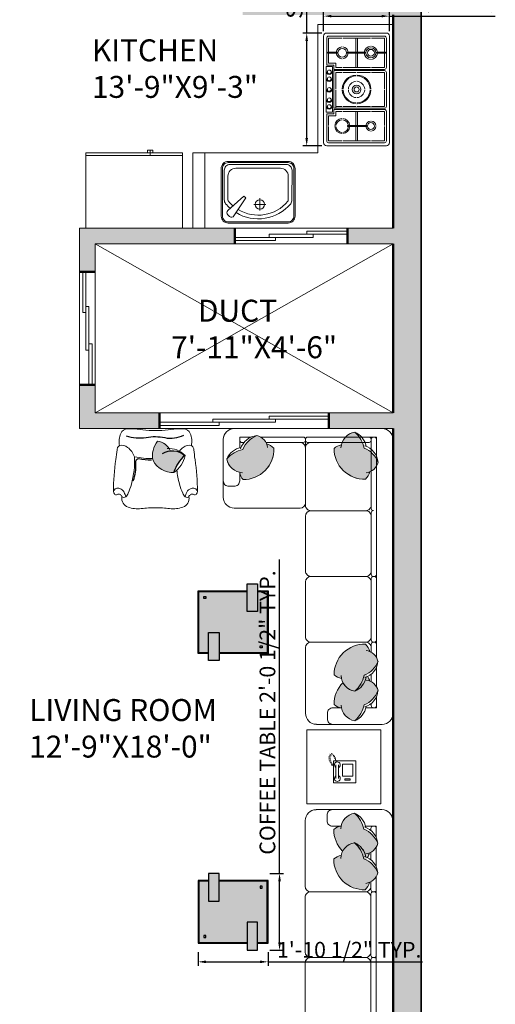
# Model space of a CAD drawing. Units: inches. Extents: x 1734 to 4011, y 1071 to 1891.
# Tile 12 of 27: x 2484 to 2636, y 1282 to 1597. Entities that reach past the tile are written whole.
import ezdxf

# ---------------------------------------------------------------- set-up
doc = ezdxf.new("R2010")
doc.units = ezdxf.units.IN
for name, color, linetype, lineweight in [('A-ANNO-DIMS', 2, 'Continuous', 18), ('A-AREA-IDEN', 3, 'Continuous', 18), ('A-EQPM', 8, 'Continuous', 18), ('A-FLOR-FIXT', 9, 'Continuous', 18), ('A-FURN', 8, 'Continuous', 18), ('A-FURN-PATT', 252, 'Continuous', 13), ('A-GLAZ', 4, 'Continuous', 18), ('A-WALL', 7, 'Continuous', 50), ('A-WALL-PATT', 8, 'Continuous', 13), ('C-PROP', 1, 'Continuous', 35)]:
    doc.layers.add(name, color=color, linetype=linetype, lineweight=lineweight)
doc.layers.add('IFF-FURN-DETAIL', color=250, linetype='Continuous')
doc.layers.add('MOBIL', color=7, linetype='Continuous')
doc.styles.get("Standard").update_dxf_attribs({"font": 'arial.ttf'})
doc.dimstyles.new('ISO-25', dxfattribs={"dimtxt": 5, "dimasz": 2.5, "dimexe": 1.25, "dimexo": 0.625, "dimtad": 1, "dimdec": 1, "dimlunit": 3, "dimtxsty": 'Standard', "dimcen": 2.5, "dimclrt": 1, "dimadec": 0, "dimazin": 0, "dimtfac": 1, "dimtdec": 1, "dimtmove": 0, "dimatfit": 3, "dimfxl": 1, "dimarcsym": 0})

# ---------------------------------------------------------------- blocks, each defined once
blk = doc.blocks.new('STOVE')
for p, q in [((11.85, 19.7), (11.55, 19.7)), ((11.55, 16.92), (11.55, 19.7)), ((11.85, 16.92), (11.85, 19.7)), ((11.85, 16.92), (11.55, 16.92)), ((-11.85, 13.73), (-11.85, 7.62)), ((-11.85, 13.73), (-11.55, 13.73)), ((-11.55, 13.73), (-11.55, 7.62)), ((11.85, 13.23), (11.55, 13.23)), ((11.55, 13.23), (11.55, 7.57)), ((11.85, 13.23), (11.85, 7.57)), ((-11.85, 10.75), (-16.4, 10.75)), ((-11.85, 10.25), (-16.4, 10.25)), ((-7, 10.75), (-11.55, 10.75)), ((-7, 10.25), (-11.55, 10.25)), ((7, 10.75), (11.55, 10.75)), ((7, 10.25), (11.55, 10.25)), ((11.85, 10.75), (16.4, 10.75)), ((11.85, 10.25), (16.4, 10.25)), ((-11.85, 7.62), (-11.55, 7.62)), ((11.85, 7.57), (11.55, 7.57)), ((-7, 3.9), (-8.4, 3.9)), ((-7.8, 3.3), (-7.8, 1)), ((-6.4, 3.3), (-7.8, 3.3)), ((-5.4, 3.9), (-6, 3.9)), ((-5.4, 3.9), (-0.15, 3.9)), ((0.15, 3.9), (5.4, 3.9)), ((6.4, 3.3), (7.8, 3.3)), ((7, 3.9), (8.4, 3.9)), ((7.8, 3.3), (7.8, 1)), ((8.4, 3.9), (8.4, 1.6)), ((11.85, 4.28), (11.55, 4.28)), ((11.55, 4.28), (11.55, 1.3)), ((11.85, 4.28), (11.85, 1.3)), ((7.3, 2.8), (-7.3, 2.8)), ((-7.3, 2.8), (-7.3, 0.8)), ((7.3, 0.8), (-7.3, 0.8)), ((7.3, 2.8), (7.3, 0.8)), ((11.85, 1.3), (11.55, 1.3))]:
    blk.add_line(p, q)
for points in [[(-17, 21), (17, 21, -0.414214), (18, 20), (18, 1, -0.414214), (17, 0), (-17, 0, -0.414214), (-18, 1), (-18, 20, -0.414214)], [(6, 3.3), (-6, 3.3), (-6, 19.4, -0.414214), (-5.4, 20), (5.4, 20, -0.414214), (6, 19.4)]]:
    blk.add_lwpolyline(points, format="xyb", close=True)
for points in [[(-7.8, 1), (-16.4, 1, -0.414214), (-17, 1.6), (-17, 19.4, -0.414214), (-16.4, 20), (-7, 20, -0.414214), (-6.4, 19.4), (-6.4, 3.3)], [(6.4, 19.4, -0.414214), (7, 20), (16.4, 20, -0.414214), (17, 19.4), (17, 1.6, -0.414214), (16.4, 1), (7.8, 1)]]:
    blk.add_lwpolyline(points, format="xyb")
for points in [[(-16.4, 15.22), (-16.4, 19.4), (-11.85, 19.4)], [(-11.55, 19.4), (-7, 19.4), (-7, 15.22)], [(-5.4, 15.22), (-5.4, 19.4), (-0.15, 19.4)], [(0.15, 19.4), (5.4, 19.4), (5.4, 15.22)], [(6.4, 3.3), (6.4, 19.4)], [(7, 15.22), (7, 19.4), (11.55, 19.4)], [(11.85, 19.4), (16.4, 19.4), (16.4, 15.22)], [(-16.4, 6.08), (-16.4, 14.92)], [(-7, 14.92), (-7, 6.08)], [(-5.4, 10.65), (-5.4, 14.92)], [(5.4, 14.92), (5.4, 10.65)], [(7, 6.08), (7, 14.92)], [(16.4, 14.92), (16.4, 6.08)], [(-5.4, 6.08), (-5.4, 10.35)], [(5.4, 10.35), (5.4, 6.08)], [(-11.85, 1.6), (-16.4, 1.6), (-16.4, 5.77)], [(-8.4, 3.9), (-8.4, 1.6), (-11.55, 1.6)], [(-7, 5.77), (-7, 3.9)], [(-5.4, 3.9), (-5.4, 5.77)], [(5.4, 5.77), (5.4, 3.9)], [(7, 3.9), (7, 5.77)], [(16.4, 5.77), (16.4, 1.6), (11.85, 1.6)], [(11.55, 1.6), (8.4, 1.6)]]:
    blk.add_lwpolyline(points)
for centre, radius in [((-11.7, 15.07), 1.1), ((11.7, 15.07), 1.6), ((11.7, 15.07), 1.1), ((0, 10.5), 1.4), ((0, 10.5), 0.8), ((11.7, 5.93), 1.4), ((-5.49, 1.8), 0.6), ((-3.3, 1.8), 0.6), ((0, 1.8), 0.6), ((3.39, 1.8), 0.6), ((5.57, 1.8), 0.6)]:
    blk.add_circle(centre, radius)
for centre, radius, start, end in [((-11.7, 15.07), 1.6, 95.3794, 174.6206), ((-11.7, 15.07), 1.6, 5.3794, 84.6206), ((11.7, 15.07), 2.1, 94.096, 175.904), ((11.7, 15.07), 2.1, 4.096, 85.904), ((-11.7, 15.07), 1.6, 185.3794, 264.6206), ((-11.7, 15.07), 1.6, 275.3794, 354.6206), ((0, 10.5), 4.6, 91.8687, 178.1313), ((0, 10.5), 4.3, 91.9991, 178.0009), ((0, 10.5), 2.6, 93.3074, 176.6926), ((0, 10.5), 4.6, 1.8687, 88.1313), ((0, 10.5), 4.3, 1.9991, 88.0009), ((0, 10.5), 2.6, 3.3074, 86.6926), ((11.7, 15.07), 2.1, 184.096, 265.904), ((11.7, 15.07), 2.1, 274.096, 355.904), ((0, 10.5), 4.6, 181.8687, 268.1313), ((0, 10.5), 4.3, 181.9991, 268.0009), ((0, 10.5), 2.6, 183.3074, 266.6926), ((0, 10.5), 4.6, 271.8687, 358.1313), ((0, 10.5), 4.3, 271.9991, 358.0009), ((0, 10.5), 2.6, 273.3074, 356.6926), ((-11.7, 5.93), 2.4, 93.5833, 176.4167), ((-11.7, 5.93), 2, 94.3012, 175.6988), ((-11.7, 5.93), 2.4, 3.5833, 86.4167), ((-11.7, 5.93), 2, 4.3012, 85.6988), ((11.7, 5.93), 1.9, 94.5281, 175.4719), ((11.7, 5.93), 1.9, 4.5281, 85.4719), ((-11.7, 5.93), 2.4, 183.5833, 266.4167), ((-11.7, 5.93), 2, 184.3012, 265.6988), ((-11.7, 5.93), 2.4, 273.5833, 356.4167), ((-11.7, 5.93), 2, 274.3012, 355.6988), ((11.7, 5.93), 1.9, 184.5281, 265.4719), ((11.7, 5.93), 1.9, 274.5281, 355.4719), ((-5.49, 1.8), 0.846, 89.9979, 270), ((-3.3, 1.8), 0.846, 89.9979, 270), ((0, 1.8), 0.846, 89.9979, 270), ((3.39, 1.8), 0.846, 89.9979, 270), ((5.57, 1.8), 0.846, 89.9979, 270)]:
    blk.add_arc(centre, radius, start, end)
blk = doc.blocks.new('Refrigerator-2 door - 36 in top')
for p, q in [((0, -26.999999), (36, -26.999999)), ((11, -27.999999), (11, -28.999999)), ((11, -28.999999), (13, -28.999999)), ((12, -26.999999), (12, -28.999999)), ((13, -28.999999), (13, -27.999999))]:
    blk.add_line(p, q)
blk.add_lwpolyline([(0, -27.999999), (0, 0), (36, 0), (36, -27.999999)], close=True)
blk = doc.blocks.new('Mesa de centro Cantria feeling')
at = {"layer": 'MOBIL', "ltscale": 0.2}
h = blk.add_hatch(color=256, dxfattribs=at)
h.set_gradient(color1=(74, 55, 38), color2=(104, 77, 54), one_color=1, tint=0.31, name='CYLINDER')
h.paths.add_polyline_path([(-0.85, -0.3), (-0.7, -0.3), (-0.7, 0.1), (-0.85, 0.1)])
h = blk.add_hatch(color=256, dxfattribs=at)
h.set_gradient(color1=(221, 221, 223), one_color=1, tint=1)
h.paths.add_polyline_path([(-0.15, -0.6), (-0.15, -0.89), (-0.01, -0.89), (-0.01, -0.01), (-0.7, -0.01), (-0.7, -0.3), (-0.85, -0.3), (-0.85, -0.01), (-0.99, -0.01), (-0.99, -0.89), (-0.3, -0.89), (-0.3, -0.6)])
h.paths.add_polyline_path([(-0.112, -0.112), (-0.112, -0.082), (-0.082, -0.082), (-0.082, -0.112)], flags=16)
h.paths.add_polyline_path([(-0.888, -0.788), (-0.888, -0.818), (-0.918, -0.818), (-0.918, -0.788)], flags=16)
h = blk.add_hatch(color=256, dxfattribs=at)
h.set_gradient(color1=(74, 55, 38), color2=(104, 77, 54), one_color=1, tint=0.31, name='CYLINDER')
h.paths.add_polyline_path([(-0.15, -0.6), (-0.3, -0.6), (-0.3, -1), (-0.15, -1)])
for points in [[(-0.85, 0), (-1, 0), (-1, -0.9), (-0.3, -0.9)], [(-0.15, -0.9), (0, -0.9), (0, 0), (-0.7, 0)], [(-0.85, -0.01), (-0.99, -0.01), (-0.99, -0.89), (-0.3, -0.89)], [(-0.15, -0.89), (-0.01, -0.89), (-0.01, -0.01), (-0.7, -0.01)]]:
    blk.add_lwpolyline(points, dxfattribs=at)
for points in [[(-0.85, -0.3), (-0.7, -0.3), (-0.7, 0.1), (-0.85, 0.1)], [(-0.082, -0.082), (-0.112, -0.082), (-0.112, -0.112), (-0.082, -0.112)], [(-0.15, -0.6), (-0.3, -0.6), (-0.3, -1), (-0.15, -1)], [(-0.918, -0.818), (-0.888, -0.818), (-0.888, -0.788), (-0.918, -0.788)]]:
    blk.add_lwpolyline(points, close=True, dxfattribs=at)
blk = doc.blocks.new('SOFA 1')
at = {"transparency": 33554687}
h = blk.add_hatch(color=256, dxfattribs=at)
h.dxf.hatch_style = 1
h.paths.add_polyline_path([(3723.52, 1308.63, 0.147724), (3717.76, 1305.24, 0.310469), (3722.42, 1300.4), (3722.42, 1300.25, 0.156703), (3723.62, 1297.8, 0.425821), (3734.69, 1309.08, 0.121928), (3732.05, 1310.63, 0.233216), (3728.6, 1313.59, 0.213835)])
h = blk.add_hatch(color=256, dxfattribs=at)
h.dxf.hatch_style = 1
h.paths.add_polyline_path([(3769.65, 1307.6, 0.084911), (3767.15, 1309.12, 0.046133), (3766.46, 1311.13), (3759.18, 1311.13, 0.039409), (3758.92, 1310.24, 0.165523), (3756.31, 1309.02, 0.42585), (3767.59, 1297.95, 0.121928), (3769.15, 1300.58, 0.027403), (3769.65, 1300.83)])
h.paths.add_polyline_path([(3765.34, 1313.08), (3760.4, 1313.08, 0.097704), (3759.18, 1311.13), (3766.46, 1311.13, 0.04873)])
h.paths.add_polyline_path([(3763.76, 1314.88, 0.16488), (3760.4, 1313.08), (3765.34, 1313.08, 0.051917)])
h.paths.add_polyline_path([(3771.6, 1305.17, 0.090388), (3769.65, 1307.6), (3769.65, 1300.83, 0.136035), (3771.6, 1302.77)])
h = blk.add_hatch(color=256, dxfattribs=at)
h.dxf.hatch_style = 1
h.paths.add_polyline_path([(3769.16, 1235.96, 0.122267), (3767.6, 1238.61, 0.425972), (3756.32, 1227.54, 0.165563), (3758.93, 1226.32, 0.309481), (3763.76, 1221.69, 0.002677), (3763.83, 1221.72, 0.146094), (3767.16, 1227.43, 0.212433), (3772.1, 1232.48, 0.235342)])
h = blk.add_hatch(color=256, dxfattribs=at)
h.dxf.hatch_style = 1
h.paths.add_polyline_path([(3769.16, 1225.36, 0.122267), (3767.6, 1228.01, 0.425972), (3756.32, 1216.94, 0.165563), (3758.93, 1215.72, 0.309481), (3763.76, 1211.09, 0.002677), (3763.83, 1211.12, 0.146094), (3767.16, 1216.83, 0.212433), (3772.1, 1221.88, 0.235342)])
for p, q in [((3720.45, 1316.13), (3773.58, 1316.13)), ((3777.51, 1312.19), (3777.51, 1213.72))]:
    blk.add_line(p, q, dxfattribs=at)
for points in [[(3717.76, 1305.24, -0.147724), (3723.52, 1308.63, -0.213355), (3728.59, 1313.59, 0.213355), (3723.52, 1308.63, 0.147724), (3717.76, 1305.24, -0.249545), (3722.86, 1309.34, 0.249545), (3717.75, 1305.25, 0.356779), (3723.4, 1300.28, -0.356779), (3717.76, 1305.24)], [(3728.58, 1313.6, -0.306333), (3732.42, 1309.31, 0.306333), (3728.58, 1313.6, 0.306674), (3722.72, 1308.89, -0.306674), (3728.58, 1313.6)], [(3763.76, 1314.88, -0.147724), (3767.15, 1309.12, -0.213355), (3772.1, 1304.05, 0.213355), (3767.15, 1309.12, 0.147724), (3763.76, 1314.88, -0.249545), (3767.86, 1309.77, 0.249545), (3763.77, 1314.89, 0.356779), (3758.8, 1309.23, -0.356779), (3763.76, 1314.88)], [(3734.69, 1309.08, -0.425972), (3723.62, 1297.8, -0.165552), (3722.4, 1300.4, 0.165552), (3723.62, 1297.79, 0.425972), (3734.69, 1309.07, 0.121514), (3732.07, 1310.63, -0.121514), (3734.69, 1309.08)], [(3767.6, 1297.95, -0.425972), (3756.31, 1309.01, -0.165552), (3758.92, 1310.24, 0.165552), (3756.31, 1309.02, 0.425972), (3767.59, 1297.95, 0.121514), (3769.14, 1300.57, -0.121514), (3767.6, 1297.95)], [(3772.11, 1304.06, -0.306333), (3767.83, 1300.22, 0.306333), (3772.11, 1304.06, 0.306674), (3767.4, 1309.91, -0.306674), (3772.11, 1304.06)], [(3770.44, 1286.63, -0.414214), (3769.66, 1287.4, 0.414214), (3770.44, 1286.63, 0.414214), (3769.66, 1285.83, -0.414214), (3770.44, 1286.63)], [(3748.01, 1262.99, -0.414214), (3746.05, 1264.95, 0.414214), (3748.01, 1262.97, 0.414213), (3746.05, 1261.01, -0.414213), (3748.01, 1262.99)], [(3770.44, 1262.99, -0.414214), (3769.66, 1263.77, 0.414214), (3770.44, 1262.99, 0.414214), (3769.66, 1262.19, -0.414214), (3770.44, 1262.99)], [(3770.83, 1262.97, -0.414214), (3771.61, 1262.19, 0.414214), (3770.83, 1262.99, 0.414214), (3771.61, 1263.77, -0.414214), (3770.83, 1262.97)], [(3748.01, 1239.35, -0.414214), (3746.05, 1241.31, 0.414214), (3748.01, 1239.33, 0.414213), (3746.05, 1237.37, -0.414213), (3748.01, 1239.35)], [(3767.7, 1239.33, -0.414214), (3769.66, 1237.37, 0.414214), (3767.7, 1239.35, 0.414214), (3769.66, 1241.31, -0.414214), (3767.7, 1239.33)], [(3770.44, 1239.35, -0.414214), (3769.66, 1240.13, 0.414214), (3770.44, 1239.33, 0.414214), (3769.66, 1238.55, -0.414214), (3770.44, 1239.35)], [(3770.83, 1239.33, -0.414214), (3771.61, 1238.55, 0.414214), (3770.83, 1239.35, 0.414214), (3771.61, 1240.13, -0.414214), (3770.83, 1239.33)], [(3756.32, 1227.54, -0.425972), (3767.6, 1238.61, -0.121514), (3769.16, 1235.98, 0.121514), (3767.6, 1238.61, 0.425972), (3756.32, 1227.54, 0.165552), (3758.93, 1226.32, -0.165552), (3756.32, 1227.54)], [(3772.1, 1232.5, -0.306674), (3767.41, 1226.64, 0.306674), (3772.1, 1232.5, 0.306333), (3767.84, 1236.34, -0.306333), (3772.1, 1232.5)], [(3763.78, 1221.67, 0.249545), (3767.87, 1226.78, -0.249545), (3763.76, 1221.69, -0.356779), (3758.81, 1227.32, 0.356779), (3763.77, 1221.68, 0.147724), (3767.16, 1227.43, 0.213355), (3772.11, 1232.51, -0.213355), (3767.16, 1227.43, -0.147724), (3763.78, 1221.67)], [(3756.32, 1216.94, -0.200233), (3759.49, 1224.76, 0.200233), (3756.32, 1216.94, 0.165552), (3758.93, 1215.72, -0.165552), (3756.32, 1216.94)], [(3772.1, 1221.9, -0.306674), (3767.41, 1216.04, 0.306674), (3772.1, 1221.9, -0.213355), (3767.16, 1216.83, -0.147724), (3763.77, 1211.08, 0.147724), (3767.15, 1216.83, 0.213355), (3772.1, 1221.9)], [(3763.76, 1211.09, -0.356779), (3758.81, 1216.72, 0.356779), (3763.76, 1211.09, 0.249545), (3767.87, 1216.18, -0.249545), (3763.76, 1211.09)]]:
    blk.add_lwpolyline(points, format="xyb", dxfattribs=at)
for points in [[(3716.51, 1312.2), (3716.51, 1291.44)], [(3722.42, 1313.08), (3722.42, 1309.23), (3722.42, 1313.08), (3726.57, 1313.08)], [(3723.21, 1311.13), (3723.93, 1311.13)], [(3729.85, 1313.08), (3745.25, 1313.08)], [(3731.82, 1311.13), (3745.25, 1311.13)], [(3746.01, 1312.3), (3746.01, 1288.55)], [(3746.01, 1310.97), (3746.01, 1311.36)], [(3768.11, 1313.08), (3746.78, 1313.08)], [(3768.87, 1311.13), (3746.78, 1311.13)], [(3771.6, 1313.08), (3767.75, 1313.08), (3771.6, 1313.08), (3771.6, 1308.93)], [(3769.66, 1287.39), (3769.65, 1312.3)], [(3771.6, 1313.08), (3771.61, 1233.74)], [(3746.01, 1288.54), (3746.01, 1308.23)], [(3769.65, 1309.43), (3769.65, 1308.71)], [(3722.42, 1300.39), (3722.42, 1297.33)], [(3720.45, 1295.38), (3718.48, 1295.38)], [(3720.45, 1287.5), (3744.09, 1287.5)], [(3747.99, 1286.6), (3767.69, 1286.6)], [(3769.66, 1263.75), (3769.66, 1285.81)], [(3746.02, 1284.63), (3746.02, 1264.94)], [(3769.66, 1277.18), (3769.66, 1263.75)], [(3746.02, 1260.99), (3746.02, 1241.3)], [(3747.99, 1262.97), (3767.69, 1262.97)], [(3769.66, 1240.12), (3769.66, 1262.18)], [(3770.43, 1262.97), (3770.82, 1262.97)], [(3747.99, 1239.33), (3767.69, 1239.33)], [(3770.43, 1239.33), (3770.82, 1239.33)], [(3746.02, 1237.36), (3746.02, 1213.74)], [(3769.66, 1235.71), (3769.66, 1238.54)], [(3771.61, 1223.14), (3771.61, 1230.47)], [(3769.66, 1225.11), (3769.66, 1227.82)], [(3767.76, 1215.72), (3771.61, 1215.72), (3771.61, 1219.84), (3771.61, 1215.72)], [(3755.86, 1215.72), (3758.92, 1215.72)], [(3769.66, 1216.5), (3769.66, 1217.22)], [(3753.91, 1211.77), (3753.91, 1213.74)], [(3749.97, 1209.8), (3773.58, 1209.8)]]:
    blk.add_lwpolyline(points, close=True, dxfattribs=at)
for points in [[(3722.42, 1311.91, 0.414214), (3723.2, 1311.13, -0.414214)], [(3770.43, 1313.08, 0.414214), (3769.65, 1312.3, -0.414214)], [(3771.6, 1312.3, 0.414214), (3770.82, 1313.08, -0.414214)], [(3716.51, 1297.34, 0.414214), (3718.47, 1295.38, -0.414214)], [(3720.44, 1295.38, 0.414214), (3722.4, 1297.34, -0.414214)], [(3716.51, 1291.45, 0.414212), (3720.44, 1287.52, -0.414212)], [(3746.03, 1288.56, 0.414214), (3747.99, 1286.6, 0.414213), (3746.03, 1284.64, -0.414213), (3747.99, 1286.6, -0.414214)], [(3769.66, 1284.64, 0.414214), (3767.7, 1286.6, 0.414214), (3769.66, 1288.56, -0.414214), (3767.7, 1286.6, -0.414214)], [(3769.66, 1261.01, 0.414214), (3767.7, 1262.97, 0.414214), (3769.66, 1264.93, -0.414214), (3767.7, 1262.97, -0.414214)], [(3772.13, 1221.9, 0.306333), (3767.84, 1225.74, -0.306333)], [(3769.16, 1225.36, 0.071861), (3768.39, 1227.01, -0.071861)], [(3755.87, 1215.72, 0.414214), (3753.91, 1213.76, -0.414214)], [(3769.66, 1216.52, 0.414214), (3770.44, 1215.74, -0.414214)], [(3770.83, 1215.74, 0.414214), (3771.61, 1216.52, -0.414214)], [(3746.05, 1213.76, 0.414212), (3749.98, 1209.82, -0.414212)], [(3755.87, 1209.8, -0.414214), (3753.91, 1211.76, 0.414214)]]:
    blk.add_lwpolyline(points, format="xyb", close=True, dxfattribs=at)
for centre, radius, start, end in [((3720.44, 1312.2), 3.93, 90.0002, 179.9998), ((3720.44, 1312.19), 3.94, 89.9158, 179.9154), ((3773.58, 1312.2), 3.93, 0.0002, 89.9998), ((3773.57, 1312.19), 3.94, 359.9158, 89.9154), ((3744.09, 1309.21), 1.92, 358.766, 90.5111), ((3745.22, 1312.29), 0.789, 0.8425, 90.8425), ((3745.24, 1311.91), 0.777, 270, 0), ((3745.24, 1311.91), 0.777, 270, 0), ((3746.8, 1312.29), 0.789, 89.1575, 179.1575), ((3746.79, 1311.91), 0.777, 180, 270), ((3746.79, 1311.91), 0.777, 180, 270), ((3747.93, 1309.21), 1.92, 89.4889, 181.234), ((3768.87, 1312.3), 0.777, 360, 90), ((3768.87, 1311.91), 0.777, 270, 0), ((3744.08, 1289.48), 1.96, 270, 360), ((3744.08, 1289.48), 1.96, 270, 360), ((3773.58, 1213.73), 3.93, 270.0002, 359.9998), ((3773.59, 1213.73), 3.93, 269.9156, 359.9152)]:
    blk.add_arc(centre, radius, start, end, dxfattribs=at)
blk = doc.blocks.new('PILLOW-1')
at = {"color": 0}
blk.add_lwpolyline([(198, -165.3, -0.232884), (126.3, -346, -0.184752), (-44.3, -233.7, -0.286563), (74.8, -22, -0.237978), (272.6, -68.2, -0.243587), (179.4, -195.4, 4.263709)], format="xyb", dxfattribs=at)
at = {"layer": 'IFF-FURN-DETAIL'}
blk.add_lwpolyline([(147.6, -117.6, -0.343333), (126.5, -342.2, 0.126408), (-39.5, -232.6, -5.969376)], format="xyb", dxfattribs=at)
blk = doc.blocks.new('CLNG90')
for points in [[(689, 370, 0.157831), (677, 385, 0.121013), (646, 395, -0.017334), (547, 407, 0.041496), (215, 431, 0.153531), (191, 423, 0.382906), (185, 395, -0.284047), (184, 361, 0.011997), (177, 351, -0.370479), (160, 345, 0.380647), (56, 282, 0.117468), (41, 146, -0.027775), (50, 0, -8.773898)], [(160, 345, 0.22481), (160, 306, 0.055398), (209, 322, 0.180116), (249, 368, 0.194833), (248, 405, 0.242377), (215, 431, 1.52074)], [(160, 345, 0.22481), (160, 306, 0.055398), (209, 322, 0.180116), (249, 368, 0.194833), (248, 405, 0.242377), (215, 431, 1.52074)], [(689, 370, -0.235486), (671, 286, -0.134038), (574, 215, -0.079303), (293, 248, -0.027048), (199, 280, -0.106276), (160, 306, -1.699)], [(689, 370, -0.235486), (671, 286, -0.134038), (574, 215, -0.079303), (293, 248, -0.027048), (199, 280, -0.106276), (160, 306, -1.699)], [(689, 370, -0.146607), (814, 357, -0.305296), (862, 286, -0.042137), (852, 131, 0.040285), (843, 0, 3.952121)], [(574, 215, 0.061244), (556, 29, 3.376255)], [(574, 215, 0.061244), (556, 29, 3.376255)], [(689, -370, -0.157831), (677, -385, -0.121013), (646, -395, 0.017334), (547, -407, -0.041496), (215, -431, -0.153531), (191, -423, -0.382906), (185, -395, 0.284047), (184, -361, -0.011997), (177, -351, 0.370479), (160, -345, -0.380647), (56, -282, -0.117468), (41, -146, 0.027775), (50, 0, 8.773898)], [(689, -370, 0.146607), (814, -357, 0.305296), (862, -286, 0.042137), (852, -131, -0.040285), (843, 0, -3.952121)], [(437, -220, 0.041086), (293, -248, 0.027048), (199, -280, 0.106276), (160, -306, 1.699)], [(437, -220, 0.041086), (293, -248, 0.027048), (199, -280, 0.106276), (160, -306, 1.699)], [(689, -370, 0.235486), (671, -286, 0.060693), (632, -247, 0.001296)], [(689, -370, 0.235486), (671, -286, 0.060693), (632, -247, 0.001296)], [(160, -345, -0.22481), (160, -306, -0.055398), (209, -322, -0.180116), (249, -368, -0.194833), (248, -405, -0.242377), (215, -431, -1.52074)], [(160, -345, -0.22481), (160, -306, -0.055398), (209, -322, -0.180116), (249, -368, -0.194833), (248, -405, -0.242377), (215, -431, -1.52074)]]:
    blk.add_lwpolyline(points, format="xyb")
at = {"layer": 'IFF-FURN-DETAIL'}
for points in [[(328, 228, 0.109125), (508, 203, -0.16587), (546, 194, -0.314359), (555, 172, 0.072017), (544, 42, 4.351186)], [(328, 228, 0.109125), (508, 203, -0.16587), (546, 194, -0.314359), (555, 172, 0.072017), (544, 42, 4.351186)], [(791, 301, 0.124986), (774, 96, -0.091334), (771, -95, 0.164688), (797, -292, 1.068868)], [(791, 301, 0.124986), (774, 96, -0.091334), (771, -95, 0.164688), (797, -292, 1.068868)]]:
    blk.add_lwpolyline(points, format="xyb", dxfattribs=at)
at = {"xscale": 1.016, "yscale": 1.016, "zscale": 1.016}
blk.add_blockref('PILLOW-1', (458, 47), dxfattribs=at)
blk.add_blockref('PILLOW-1', (458, 47), dxfattribs=at)
blk = doc.blocks.new('*D81')
at = {"layer": 'A-ANNO-DIMS', "color": 0, "lineweight": -2, "transparency": 16777216}
for p, q in [((2567.27, 1324.11), (2567.27, 1424.27)), ((2564.22, 1324.11), (2568.52, 1324.11)), ((2567.27, 1302.06), (2567.27, 1321.61)), ((2564.22, 1299.56), (2568.52, 1299.56))]:
    blk.add_line(p, q, dxfattribs=at)
at = {"layer": 'A-ANNO-DIMS', "color": 0, "transparency": 16777216}
for points in [[(2566.86, 1321.61), (2567.69, 1321.61), (2567.27, 1324.11)], [(2566.86, 1302.06), (2567.69, 1302.06), (2567.27, 1299.56)]]:
    blk.add_solid(points, dxfattribs=at)
at = {"layer": 'Defpoints', "color": 0, "transparency": 16777216}
for p in [(2563.59, 1324.11), (2567.27, 1324.11), (2563.59, 1299.56)]:
    blk.add_point(p, dxfattribs=at)
at = {"layer": 'A-ANNO-DIMS', "color": 1, "transparency": 16777216, "insert": (2564.06, 1375.44), "char_height": 5, "attachment_point": 5, "rotation": 90}
blk.add_mtext('COFFEE TABLE 2\'-0 1/2" TYP.', dxfattribs=at)
blk = doc.blocks.new('*D82')
at = {"layer": 'A-ANNO-DIMS', "color": 0, "lineweight": -2, "transparency": 16777216}
for p, q in [((2541.28, 1298.94), (2541.28, 1294.63)), ((2563.59, 1298.94), (2563.59, 1294.63)), ((2543.78, 1295.88), (2561.09, 1295.88)), ((2563.59, 1295.88), (2612.88, 1295.88))]:
    blk.add_line(p, q, dxfattribs=at)
at = {"layer": 'A-ANNO-DIMS', "color": 0, "transparency": 16777216}
for points in [[(2543.78, 1296.3), (2543.78, 1295.46), (2541.28, 1295.88)], [(2561.09, 1296.3), (2561.09, 1295.46), (2563.59, 1295.88)]]:
    blk.add_solid(points, dxfattribs=at)
at = {"layer": 'Defpoints', "color": 0, "transparency": 16777216}
for p in [(2541.28, 1299.56), (2563.59, 1299.56), (2563.59, 1295.88)]:
    blk.add_point(p, dxfattribs=at)
at = {"layer": 'A-ANNO-DIMS', "color": 1, "transparency": 16777216, "insert": (2589.49, 1299.09), "char_height": 5, "attachment_point": 5}
blk.add_mtext('1\'-10 1/2" TYP.', dxfattribs=at)
blk = doc.blocks.new('*D95')
at = {"layer": 'A-ANNO-DIMS', "color": 0, "lineweight": -2, "transparency": 16777216}
for p, q in [((2575.94, 1592.3), (2575.94, 1652.12)), ((2580.71, 1592.3), (2574.69, 1592.3)), ((2575.94, 1558.8), (2575.94, 1589.8)), ((2580.71, 1556.3), (2574.69, 1556.3))]:
    blk.add_line(p, q, dxfattribs=at)
at = {"layer": 'A-ANNO-DIMS', "color": 0, "transparency": 16777216}
for points in [[(2575.52, 1589.8), (2576.35, 1589.8), (2575.94, 1592.3)], [(2575.52, 1558.8), (2576.35, 1558.8), (2575.94, 1556.3)]]:
    blk.add_solid(points, dxfattribs=at)
at = {"layer": 'Defpoints', "color": 0, "transparency": 16777216}
for p in [(2575.94, 1592.3), (2581.34, 1592.3), (2581.34, 1556.3)]:
    blk.add_point(p, dxfattribs=at)
at = {"layer": 'A-ANNO-DIMS', "color": 1, "transparency": 16777216, "insert": (2572.72, 1623.46), "char_height": 5, "attachment_point": 5, "rotation": 90}
blk.add_mtext('STOVE 3\'-0" TYP.', dxfattribs=at)
blk = doc.blocks.new('*D96')
at = {"layer": 'A-ANNO-DIMS', "color": 0, "lineweight": -2, "transparency": 16777216}
for p, q in [((2581.34, 1592.93), (2581.34, 1598.95)), ((2583.84, 1597.7), (2599.84, 1597.7)), ((2602.34, 1592.93), (2602.34, 1598.95)), ((2602.34, 1597.7), (2636.09, 1597.7))]:
    blk.add_line(p, q, dxfattribs=at)
at = {"layer": 'A-ANNO-DIMS', "color": 0, "transparency": 16777216}
for points in [[(2583.84, 1598.12), (2583.84, 1597.29), (2581.34, 1597.7)], [(2599.84, 1598.12), (2599.84, 1597.29), (2602.34, 1597.7)]]:
    blk.add_solid(points, dxfattribs=at)
at = {"layer": 'Defpoints', "color": 0, "transparency": 16777216}
for p in [(2602.34, 1597.7), (2581.34, 1592.3), (2602.34, 1592.3)]:
    blk.add_point(p, dxfattribs=at)
at = {"layer": 'A-ANNO-DIMS', "color": 1, "transparency": 16777216, "insert": (2620.47, 1600.88), "char_height": 5, "attachment_point": 5}
blk.add_mtext('1\'-9" TYP.', dxfattribs=at)

msp = doc.modelspace()

# ---------------------------------------------------------------- hatches: boundary and pattern name
at = {"layer": 'A-FURN-PATT'}
h = msp.add_hatch(dxfattribs=at)
h.set_pattern_fill('ANSI32', color=256)
h.set_pattern_definition([(45, (-758.361, 0), (-6.735192, 6.735192), []), (45, (-753.871, 0), (-6.735192, 6.735192), [])])
h.paths.add_polyline_path([(2366.48, 1466.06), (2306.48, 1466.06), (2306.48, 1448.06), (2366.48, 1448.06)])
h.paths.add_polyline_path([(2310.37, 1452.28), (2359.82, 1452.28), (2359.82, 1462.58), (2310.37, 1462.58)], flags=24)
h.paths.add_polyline_path([(2525.12, 1646.17), (2525.12, 1700.88), (2499, 1700.88), (2499, 1646.17)], flags=9)
h.paths.add_polyline_path([(2555.1, 1646.17), (2555.1, 1700.88), (2528.98, 1700.88), (2528.98, 1646.17)], flags=9)
h.paths.add_polyline_path([(2492.08, 1807.82), (2546.48, 1807.82), (2546.48, 1833.94), (2492.08, 1833.94)], flags=9)
h.paths.add_polyline_path([(2464.41, 1783), (2507.08, 1783), (2507.08, 1791.24), (2464.41, 1791.24)], flags=9)
h.paths.add_polyline_path([(2467.59, 1146.53), (2480.18, 1146.53), (2480.18, 1156.83), (2467.59, 1156.83)], flags=9)
h.paths.add_polyline_path([(2467.58, 1215.53), (2479.78, 1215.53), (2479.78, 1225.83), (2467.58, 1225.83)], flags=9)
h.paths.add_polyline_path([(2292.19, 1646.17), (2292.19, 1700.88), (2266.07, 1700.88), (2266.07, 1646.17)], flags=9)
h.paths.add_polyline_path([(2504.62, 1567.64), (2559.02, 1567.64), (2559.02, 1593.76), (2504.62, 1593.76)], flags=9)
h.paths.add_polyline_path([(2562.71, 1614.15), (2583.08, 1614.15), (2583.08, 1624.45), (2562.71, 1624.45)], flags=9)
h.paths.add_polyline_path([(2522.41, 1650.28), (2571.86, 1650.28), (2571.86, 1660.58), (2522.41, 1660.58)], flags=9)
h.paths.add_polyline_path([(2504.36, 1707.67), (2564.2, 1707.67), (2564.2, 1733.79), (2504.36, 1733.79)], flags=9)
h.paths.add_polyline_path([(2381.34, 1790.51), (2430.31, 1790.51), (2430.31, 1816.63), (2381.34, 1816.63)], flags=9)
h.paths.add_polyline_path([(2291.99, 1790.51), (2340.95, 1790.51), (2340.95, 1816.63), (2291.99, 1816.63)], flags=9)
h.paths.add_polyline_path([(2330.54, 1224.14), (2390.38, 1224.14), (2390.38, 1250.26), (2330.54, 1250.26)], flags=9)
h.paths.add_polyline_path([(2425.61, 1508.95), (2480.02, 1508.95), (2480.02, 1535.07), (2425.61, 1535.07)], flags=9)
h.paths.add_polyline_path([(2505.48, 1357.1), (2574.53, 1357.1), (2574.53, 1383.22), (2505.48, 1383.22)], flags=9)
h.paths.add_polyline_path([(2530.46, 1484.55), (2584.86, 1484.55), (2584.86, 1510.67), (2530.46, 1510.67)], flags=9)
h.paths.add_polyline_path([(2349.79, 1659.95), (2415.08, 1659.95), (2415.08, 1686.07), (2349.79, 1686.07)], flags=9)
h = msp.add_hatch(color=256, dxfattribs=at)
h.dxf.hatch_style = 1
h.paths.add_polyline_path([(2533.5, 1452.07, -0.129718), (2537, 1457.46, 0.218011), (2532.44, 1459, 0.250405), (2528.37, 1462.06, 0.237978), (2526.92, 1455.83, 0.283254)])
at = {"layer": 'A-WALL-PATT'}
h = msp.add_hatch(color=256, dxfattribs=at)
h.dxf.hatch_style = 1
h.paths.add_polyline_path([(2612.48, 1844.06), (2261.48, 1844.06), (2261.48, 1758.06), (2270.05, 1758.06), (2270.05, 1763.06), (2266.48, 1763.06), (2266.48, 1835.06), (2353.48, 1835.06), (2353.48, 1793.06), (2358.48, 1793.06), (2358.48, 1835.06), (2445.48, 1835.06), (2445.48, 1763.06), (2393.48, 1763.06), (2393.48, 1758.06), (2445.48, 1758.06), (2445.48, 1617.06), (2450.48, 1617.06), (2450.48, 1641.06), (2454.48, 1641.06), (2454.48, 1646.06), (2450.48, 1646.06), (2450.48, 1790.06), (2456.52, 1790.06), (2456.52, 1799.06), (2450.48, 1799.06), (2450.48, 1839.06), (2603.48, 1839.06), (2603.48, 1799.06), (2585.48, 1799.06), (2585.48, 1790.06), (2603.48, 1790.06), (2603.48, 1646.06), (2490.48, 1646.06), (2490.48, 1641.06), (2603.48, 1641.06), (2603.48, 1601.06), (2555.48, 1601.06), (2555.48, 1598.06), (2603.48, 1598.06), (2603.48, 1530.06), (2588.98, 1530.06), (2588.98, 1525.06), (2603.48, 1525.06), (2603.48, 1471.06), (2582.98, 1471.06), (2582.98, 1466.06), (2612.48, 1466.06)])
h.paths.add_polyline_path([(2612.48, 1466.06), (2603.48, 1466.06), (2603.48, 1250.06), (2509.48, 1250.06), (2509.48, 1241.06), (2603.48, 1241.06), (2603.48, 1133.06), (2428.48, 1133.06), (2428.48, 1124.06), (2612.48, 1124.06)])
h = msp.add_hatch(color=256, dxfattribs=at)
h.dxf.hatch_style = 1
h.paths.add_polyline_path([(2503.48, 1516.06), (2508.48, 1516.06), (2508.48, 1525.06), (2552.98, 1525.06), (2552.98, 1530.06), (2503.48, 1530.06)])
h.paths.add_polyline_path([(2503.48, 1466.06), (2528.98, 1466.06), (2528.98, 1471.06), (2508.48, 1471.06), (2508.48, 1480.06), (2503.48, 1480.06)])

# ---------------------------------------------------------------- linework, layer by layer
at = {"layer": 'A-FLOR-FIXT'}
msp.add_circle((2561, 1537.61), 1.5, dxfattribs=at)
at = {"layer": 'A-FURN'}
for p, q in [((2579.48, 1595.06), (2579.48, 1554.06)), ((2579.48, 1595.06), (2603.48, 1595.06)), ((2539.66, 1554.06), (2579.48, 1554.06)), ((2539.66, 1530.06), (2539.66, 1554.06)), ((2543.48, 1554.06), (2543.48, 1530.06)), ((2503.48, 1530.06), (2603.48, 1530.06)), ((2503.48, 1530.06), (2503.48, 1466.06)), ((2508.48, 1525.06), (2603.48, 1525.06)), ((2508.48, 1525.06), (2508.48, 1471.06)), ((2508.48, 1525.06), (2603.48, 1471.06)), ((2508.48, 1471.06), (2603.48, 1525.06)), ((2508.48, 1471.06), (2603.48, 1471.06)), ((2503.48, 1466.06), (2603.48, 1466.06))]:
    msp.add_line(p, q, dxfattribs=at)
for points in [[(2550.89, 1551.33, 0.414214), (2548.65, 1549.11), (2548.67, 1533.88, 0.414214), (2550.87, 1531.64), (2570.02, 1531.66, 0.414214), (2572.24, 1533.87), (2572.24, 1549.11, 0.414214), (2570.01, 1551.33), (2550.89, 1551.33)], [(2550.89, 1550.96, 0.414214), (2549.04, 1549.11), (2549.04, 1533.88, 0.414214), (2550.87, 1532.03), (2570.02, 1532.03, 0.414214), (2571.84, 1533.87), (2571.84, 1549.11, 0.414214), (2570.01, 1550.94), (2550.89, 1550.96)], [(2553.4, 1534.99, 0.371519), (2570.83, 1537.84, 0.175764), (2571.24, 1539.02), (2571.26, 1548.51, 0.414214), (2569.41, 1550.33), (2551.49, 1550.36, 0.414214), (2549.64, 1548.5), (2549.64, 1539.02, 0.175764), (2550.07, 1537.84, 0.038632), (2551.53, 1536.36)], [(2554.06, 1535.97, 0.370401), (2569.93, 1538.6, 0.175764), (2570.06, 1539.02), (2570.06, 1546.66, 0.414214), (2567.55, 1549.15), (2553.34, 1549.15, 0.414214), (2550.83, 1546.65), (2550.83, 1539.02, 0.175764), (2550.98, 1538.6, 0.038512), (2552.42, 1537.16)]]:
    msp.add_lwpolyline(points, format="xyb", dxfattribs=at)
for points in [[(2550.76, 1534.24), (2551.34, 1533.75, 0.463205), (2552.73, 1533.96), (2556.56, 1539.69), (2555.86, 1540.29), (2550.78, 1535.65, 0.4637)], [(2586.16, 1357.94, 3.938511), (2585.28, 1357.94, -3.938511)], [(2585.28, 1355.21, 3.938511), (2586.16, 1355.21, -3.938511)]]:
    msp.add_lwpolyline(points, format="xyb", close=True, dxfattribs=at)
for points in [[(2562.94, 1537.6), (2559.04, 1537.6)], [(2560.99, 1535.65), (2560.99, 1539.55)], [(2599.6, 1369.87), (2599.6, 1346.25), (2575.99, 1346.25), (2575.99, 1369.87)]]:
    msp.add_lwpolyline(points, dxfattribs=at)
for points in [[(2575.99, 1346.25), (2575.99, 1369.87), (2599.6, 1369.87), (2599.6, 1346.25)], [(2583.18, 1361.77), (2583.69, 1361.61)], [(2583.34, 1362.12), (2583.88, 1361.96)], [(2583.76, 1362.38), (2584.27, 1362.19)], [(2584.22, 1361.96), (2584.73, 1361.77)], [(2584.73, 1360.91), (2585.25, 1360.73)], [(2583.18, 1360.06), (2583.69, 1359.87)], [(2584.48, 1360.06), (2591.58, 1360.06), (2591.58, 1353.05), (2584.48, 1353.05)], [(2591.58, 1360.06), (2591.58, 1353.05), (2584.48, 1353.05), (2584.48, 1360.06)], [(2585.08, 1360.57), (2585.38, 1359.57)], [(2585.27, 1358.73), (2585.27, 1354.4)], [(2586.13, 1358.73), (2586.13, 1354.4)], [(2590.65, 1355.18), (2587.4, 1355.18), (2587.4, 1358.99), (2590.65, 1358.99)], [(2587.4, 1355.18), (2587.4, 1358.99), (2590.65, 1358.99), (2590.65, 1355.18)], [(2589.84, 1354.23), (2589.84, 1353.84), (2588.1, 1353.84), (2588.1, 1354.23)], [(2588.1, 1354.23), (2589.84, 1354.23), (2589.84, 1353.84), (2588.1, 1353.84)]]:
    msp.add_lwpolyline(points, close=True, dxfattribs=at)
at = {"layer": 'A-GLAZ'}
for p, q in [((2563.98, 1527.06), (2563.98, 1528.06)), ((2563.98, 1528.06), (2588.98, 1528.06)), ((2575.98, 1528.06), (2575.98, 1529.06)), ((2575.98, 1529.06), (2588.98, 1529.06)), ((2577.98, 1527.06), (2577.98, 1528.06)), ((2552.98, 1527.06), (2577.98, 1527.06)), ((2552.98, 1526.06), (2565.98, 1526.06)), ((2565.98, 1526.06), (2565.98, 1527.06)), ((2504.48, 1503.06), (2504.48, 1516.06)), ((2505.48, 1491.06), (2505.48, 1516.06)), ((2505.48, 1503.06), (2504.48, 1503.06)), ((2506.48, 1505.06), (2505.48, 1505.06)), ((2506.48, 1480.06), (2506.48, 1505.06)), ((2507.48, 1493.06), (2506.48, 1493.06)), ((2507.48, 1480.06), (2507.48, 1493.06)), ((2506.48, 1491.06), (2505.48, 1491.06)), ((2528.98, 1468.06), (2565.98, 1468.06)), ((2545.98, 1469.06), (2545.98, 1468.06)), ((2545.98, 1469.06), (2582.98, 1469.06)), ((2547.98, 1468.06), (2547.98, 1467.06)), ((2563.98, 1470.06), (2563.98, 1469.06)), ((2563.98, 1470.06), (2582.98, 1470.06)), ((2565.98, 1469.06), (2565.98, 1468.06)), ((2528.98, 1467.06), (2547.98, 1467.06))]:
    msp.add_line(p, q, dxfattribs=at)
for points in [[(2583, 1361.42), (2583.53, 1361.26)], [(2583, 1361.08), (2583.53, 1360.91)], [(2583, 1360.73), (2583.53, 1360.57)], [(2584.39, 1361.61), (2584.9, 1361.42)], [(2584.55, 1361.26), (2585.08, 1361.08)], [(2583, 1360.38), (2583.53, 1360.22)], [(2583.34, 1359.71), (2583.88, 1359.52)], [(2583.53, 1359.36), (2584.04, 1359.17)], [(2583.69, 1359.01), (2584.22, 1358.83)], [(2583.88, 1358.66), (2584.39, 1358.48)]]:
    msp.add_lwpolyline(points, close=True, dxfattribs=at)
at = {"layer": 'A-WALL'}
for p, q in [((2603.48, 1598.06), (2603.48, 1530.06)), ((2552.98, 1525.06), (2552.98, 1530.06)), ((2588.98, 1525.06), (2588.98, 1530.06)), ((2603.48, 1525.06), (2603.48, 1471.06)), ((2508.48, 1516.06), (2503.48, 1516.06)), ((2508.48, 1480.06), (2503.48, 1480.06)), ((2528.98, 1471.06), (2528.98, 1466.06)), ((2582.98, 1471.06), (2582.98, 1466.06)), ((2603.48, 1466.06), (2603.48, 1250.06))]:
    msp.add_line(p, q, dxfattribs=at)
at = {"layer": 'C-PROP'}
msp.add_lwpolyline([(2428.48, 1124.06), (2252.48, 1124.06), (2252.48, 1844.06), (2612.48, 1844.06), (2612.48, 1124.06), (2428.48, 1124.06)], dxfattribs=at)

# ---------------------------------------------------------------- block references
at = {"layer": 'A-EQPM', "xscale": -1, "rotation": 270}
msp.add_blockref('STOVE', (2581.34, 1574.3), dxfattribs=at)
at = {"layer": 'A-EQPM', "xscale": 0.8569942030484906, "yscale": 0.8569942030484906, "zscale": 0.8569942030484906, "rotation": 180}
msp.add_blockref('Refrigerator-2 door - 36 in top', (2536.33, 1530.06), dxfattribs=at)
at = {"layer": 'A-FURN'}
for name, p, xscale, yscale, zscale, rotation in [('CLNG90', (2527.69, 1439.27), 0.031001591544, 0.031001591544, 0.031001591544, 90), ('Mesa de centro Cantria feeling', (2563.59, 1394.25), -22.3138190187957, 22.3138190187957, 22.3138190187957, 180), ('SOFA 1', (-749.74, 2418.33), -0.887653230693335, 0.887653230693335, 0.887653230693335, 180)]:
    msp.add_blockref(name, p, dxfattribs=dict(at, xscale=xscale, yscale=yscale, zscale=zscale, rotation=rotation))
for name, p, xscale, yscale, zscale in [('SOFA 1', (-749.64, 297.79), 0.887653230693335, 0.887653230693335, 0.887653230693335), ('Mesa de centro Cantria feeling', (2563.59, 1321.88), 22.3138190187957, 22.3138190187957, 22.3138190187957)]:
    msp.add_blockref(name, p, dxfattribs=dict(at, xscale=xscale, yscale=yscale, zscale=zscale))

# ---------------------------------------------------------------- texts
at = {"layer": 'A-AREA-IDEN', "char_height": 7, "attachment_point": 1}
for s, insert in [('KITCHEN\\P13\'-9"X9\'-3"', (2507.43, 1590.28)), ('    DUCT\\P7\'-11"X4\'-6"', (2532.67, 1507.18)), ('LIVING ROOM\\P12\'-9"X18\'-0"', (2487.41, 1379.74))]:
    msp.add_mtext_dynamic_manual_height_columns(s, width=86.9528, gutter_width=12.5, heights=[0], dxfattribs=dict(at, insert=insert))

# ---------------------------------------------------------------- dimensions: what is measured, and where the dimension line sits
at = {"layer": 'A-ANNO-DIMS'}
for base, p1, p2, text, picture, middle in [((2575.94, 1592.3), (2581.34, 1556.3), (2581.34, 1592.3), 'STOVE <> TYP.', '*D95', (2572.72, 1623.46)), ((2567.2736, 1324.1069), (2563.5918, 1299.5617), (2563.5918, 1324.1069), 'COFFEE TABLE <> TYP.', '*D81', (2564.0616, 1375.4362))]:
    dim = msp.add_linear_dim(base=base, p1=p1, p2=p2, angle=90, text=text, dimstyle='ISO-25', override={"dimdec": 1, "dimrnd": 0, "dimzin": 1, "dimlunit": 4, "dimfrac": 2}, dxfattribs=at)
    dim.commit()
    dim.dimension.update_dxf_attribs({"geometry": picture, "text_midpoint": middle})
for base, p1, p2, picture, middle in [((2602.34, 1597.7), (2581.34, 1592.3), (2602.34, 1592.3), '*D96', (2620.47, 1600.88)), ((2563.59, 1295.88), (2541.28, 1299.56), (2563.59, 1299.56), '*D82', (2589.49, 1299.09))]:
    dim = msp.add_linear_dim(base=base, p1=p1, p2=p2, text='<> TYP.', dimstyle='ISO-25', override={"dimdec": 1, "dimrnd": 0, "dimzin": 1, "dimlunit": 4, "dimfrac": 2}, dxfattribs=at)
    dim.commit()
    dim.dimension.update_dxf_attribs({"geometry": picture, "text_midpoint": middle})

doc.saveas('drawing.dxf')
